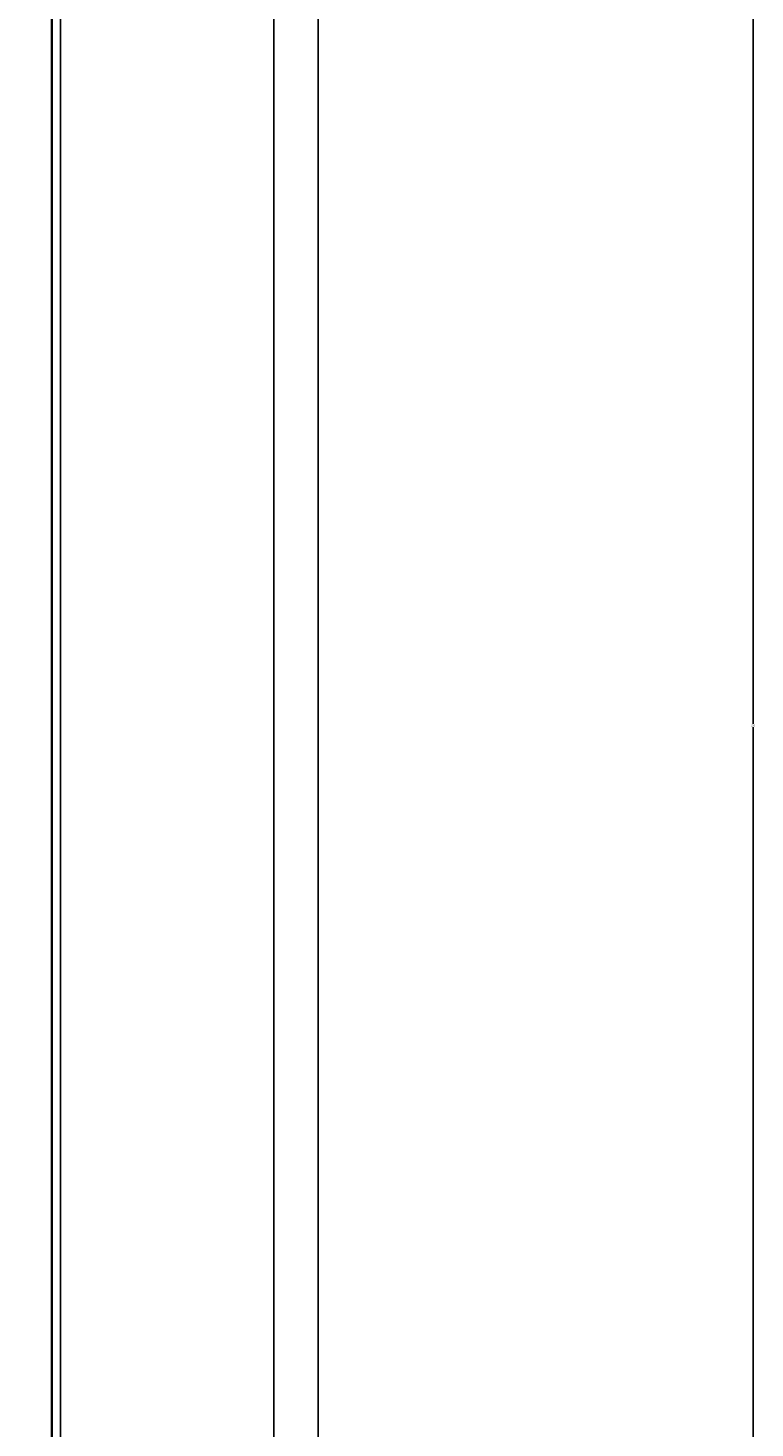
# Model space of a CAD drawing. Units: inches. Extents: x 3731 to 4318, y 1310 to 2388.
# Tile 22 of 57: x 4237 to 4318, y 1397 to 1554. Entities that reach past the tile are written whole.
import ezdxf

# ---------------------------------------------------------------- set-up
doc = ezdxf.new("R2010")
doc.units = ezdxf.units.IN
doc.layers.add('A-ANNO-DIMS', color=2, linetype='Continuous', lineweight=18)
doc.layers.add('A-WALL', color=7, linetype='Continuous', lineweight=35)
doc.styles.get("Standard").update_dxf_attribs({"font": 'arial.ttf'})
doc.dimstyles.get("Standard").update_dxf_attribs({"dimtxt": 0.18, "dimasz": 0.18, "dimexe": 0.18, "dimexo": 0.0625, "dimgap": 0.09, "dimtad": 0, "dimtih": 1, "dimtoh": 1, "dimdec": 4, "dimzin": 0, "dimdsep": 46, "dimtxsty": 'Standard', "dimcen": 0.09, "dimadec": 0, "dimazin": 0, "dimtfac": 1, "dimtdec": 4, "dimtofl": 0, "dimtmove": 0, "dimatfit": 3, "dimfxl": 1, "dimtolj": 1, "dimtzin": 0, "dimarcsym": 0})

# ---------------------------------------------------------------- blocks, each defined once
blk = doc.blocks.new('*D32')
at = {"layer": 'A-ANNO-DIMS', "color": 0, "lineweight": -2, "transparency": 16777216}
for p, q in [((4269.21, 1592.32), (4269.21, 1310.25)), ((3835.21, 1359.32), (3835.21, 1310.25)), ((3835.39, 1310.43), (4051.92, 1310.43)), ((4269.03, 1310.43), (4052.5, 1310.43))]:
    blk.add_line(p, q, dxfattribs=at)
at = {"layer": 'A-ANNO-DIMS', "color": 0, "transparency": 16777216}
for points in [[(3835.39, 1310.46), (3835.39, 1310.4), (3835.21, 1310.43)], [(4269.03, 1310.46), (4269.03, 1310.4), (4269.21, 1310.43)]]:
    blk.add_solid(points, dxfattribs=at)
at = {"layer": 'Defpoints', "color": 0, "transparency": 16777216}
for p in [(4269.21, 1592.38), (3835.21, 1359.38), (4269.21, 1310.43)]:
    blk.add_point(p, dxfattribs=at)
at = {"layer": 'A-ANNO-DIMS', "color": 0, "transparency": 16777216, "insert": (4052.21, 1310.43), "char_height": 0.18, "attachment_point": 5}
blk.add_mtext('\\A1;434', dxfattribs=at)
blk = doc.blocks.new('*D42')
at = {"layer": 'A-ANNO-DIMS', "color": 0, "lineweight": -2, "transparency": 16777216}
for p, q in [((4269.27, 1592.38), (4318.34, 1592.38)), ((4318.16, 1592.2), (4318.16, 1476.06)), ((4318.16, 1359.56), (4318.16, 1475.7)), ((4239.27, 1359.38), (4318.34, 1359.38))]:
    blk.add_line(p, q, dxfattribs=at)
at = {"layer": 'A-ANNO-DIMS', "color": 0, "transparency": 16777216}
for points in [[(4318.13, 1592.2), (4318.19, 1592.2), (4318.16, 1592.38)], [(4318.13, 1359.56), (4318.19, 1359.56), (4318.16, 1359.38)]]:
    blk.add_solid(points, dxfattribs=at)
at = {"layer": 'Defpoints', "color": 0, "transparency": 16777216}
for p in [(4269.21, 1592.38), (4318.16, 1592.38), (4239.21, 1359.38)]:
    blk.add_point(p, dxfattribs=at)
at = {"layer": 'A-ANNO-DIMS', "color": 0, "transparency": 16777216, "insert": (4318.16, 1475.88), "char_height": 0.18, "attachment_point": 5}
blk.add_mtext('\\A1;233', dxfattribs=at)
blk = doc.blocks.new('*D43')
at = {"layer": 'A-ANNO-DIMS', "color": 0, "lineweight": -2, "transparency": 16777216}
for p, q in [((4240.21, 1597.39), (4240.21, 1310.25)), ((4264.21, 1597.32), (4264.21, 1310.25)), ((4240.39, 1310.43), (4251.99, 1310.43)), ((4264.03, 1310.43), (4252.43, 1310.43))]:
    blk.add_line(p, q, dxfattribs=at)
at = {"layer": 'A-ANNO-DIMS', "color": 0, "transparency": 16777216}
for points in [[(4240.39, 1310.46), (4240.39, 1310.4), (4240.21, 1310.43)], [(4264.03, 1310.46), (4264.03, 1310.4), (4264.21, 1310.43)]]:
    blk.add_solid(points, dxfattribs=at)
at = {"layer": 'Defpoints', "color": 0, "transparency": 16777216}
for p in [(4240.21, 1597.45), (4264.21, 1597.38), (4264.21, 1310.43)]:
    blk.add_point(p, dxfattribs=at)
at = {"layer": 'A-ANNO-DIMS', "color": 0, "transparency": 16777216, "insert": (4252.21, 1310.43), "char_height": 0.18, "attachment_point": 5}
blk.add_mtext('\\A1;24', dxfattribs=at)

msp = doc.modelspace()

# ---------------------------------------------------------------- linework, layer by layer
at = {"layer": 'A-WALL'}
msp.add_line((4239.21, 1592.38), (4239.21, 1359.38), dxfattribs=at)

# ---------------------------------------------------------------- dimensions: what is measured, and where the dimension line sits
at = {"layer": 'A-ANNO-DIMS'}
for base, p1, p2, picture, middle in [((4264.21, 1310.43), (4240.21, 1597.45), (4264.21, 1597.38), '*D43', (4252.21, 1310.43)), ((4269.21, 1310.43), (3835.21, 1359.38), (4269.21, 1592.38), '*D32', (4052.21, 1310.43))]:
    dim = msp.add_linear_dim(base=base, p1=p1, p2=p2, dimstyle='Standard', override={"dimdec": 0, "dimlfac": 1, "dimrnd": 0, "dimzin": 0, "dimdsep": 46, "dimlunit": 2}, dxfattribs=at)
    dim.commit()
    dim.dimension.update_dxf_attribs({"geometry": picture, "text_midpoint": middle})
dim = msp.add_linear_dim(base=(4318.16, 1592.38), p1=(4239.21, 1359.38), p2=(4269.21, 1592.38), angle=90, dimstyle='Standard', override={"dimdec": 0, "dimlfac": 1, "dimrnd": 0, "dimzin": 0, "dimdsep": 46, "dimlunit": 2}, dxfattribs=at)
dim.commit()
dim.dimension.update_dxf_attribs({"geometry": '*D42', "text_midpoint": (4318.16, 1475.88)})

doc.saveas('drawing.dxf')
